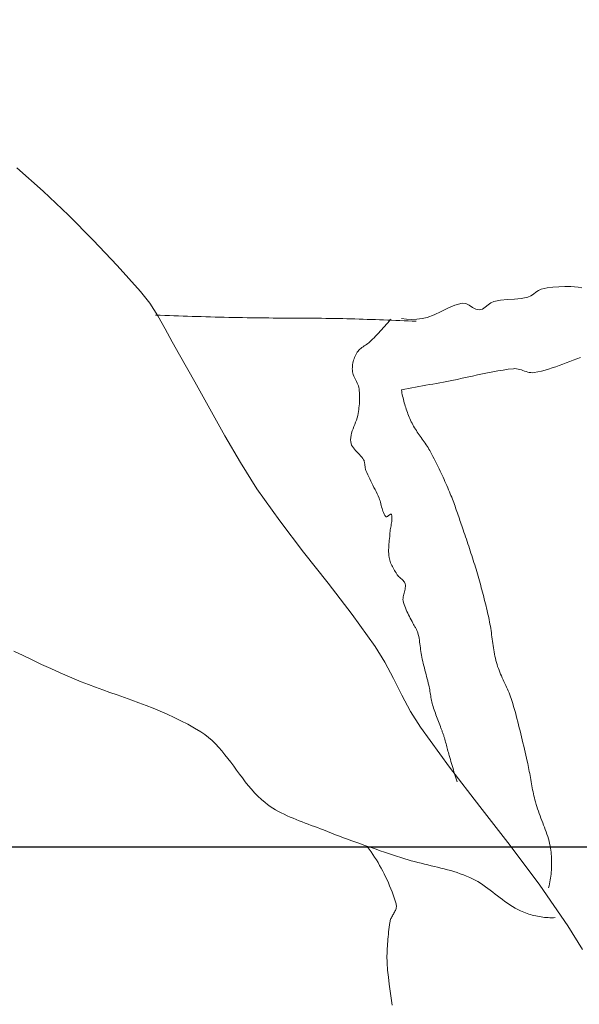
# Model space of a CAD drawing. Units: inches. Extents: x 1484 to 2008, y 1843 to 2590.
# Tile 7 of 21: x 1853 to 1872, y 2005 to 2039. Entities that reach past the tile are written whole.
import ezdxf

# ---------------------------------------------------------------- set-up
doc = ezdxf.new("R2010")
doc.units = ezdxf.units.IN
doc.layers.add('A-ANNO-DIMS', color=2, linetype='Continuous', lineweight=18)
doc.layers.add('A-FURN', color=8, linetype='Continuous', lineweight=18)
doc.styles.get("Standard").update_dxf_attribs({"font": 'arial.ttf'})
doc.dimstyles.new('ISO-25', dxfattribs={"dimtxt": 7, "dimasz": 2.5, "dimexe": 1.25, "dimexo": 0.625, "dimtad": 1, "dimdec": 0, "dimlunit": 3, "dimtxsty": 'Standard', "dimcen": 2.5, "dimadec": 0, "dimazin": 0, "dimtfac": 1, "dimtdec": 0, "dimtmove": 0, "dimatfit": 3, "dimfxl": 1, "dimarcsym": 0})

# ---------------------------------------------------------------- blocks, each defined once
blk = doc.blocks.new('BED-DOUBLE')
for p, q in [((4.353, 67.391), (4.375, 67.517)), ((27.04, 67.54), (26.237, 67.038)), ((4.326, 67.139), (4.333, 67.265)), ((4.331, 66.934), (4.326, 67.139)), ((4.333, 67.265), (4.353, 67.391)), ((6.802, 67.342), (6.757, 67.462)), ((6.847, 67.221), (6.802, 67.342)), ((6.893, 67.101), (6.847, 67.221)), ((4.338, 66.728), (4.331, 66.934)), ((6.939, 66.981), (6.893, 67.101)), ((6.985, 66.86), (6.939, 66.981)), ((7.03, 66.739), (6.985, 66.86)), ((26.237, 67.038), (24.84, 66.077)), ((4.352, 66.524), (4.338, 66.728)), ((4.377, 66.32), (4.352, 66.524)), ((7.073, 66.618), (7.03, 66.739)), ((7.115, 66.496), (7.073, 66.618)), ((7.154, 66.374), (7.115, 66.496)), ((23.776, 66.463), (23.709, 66.456)), ((23.844, 66.468), (23.776, 66.463)), ((23.912, 66.472), (23.844, 66.468)), ((23.981, 66.475), (23.912, 66.472)), ((24.049, 66.476), (23.981, 66.475)), ((24.117, 66.476), (24.049, 66.476)), ((24.186, 66.475), (24.117, 66.476)), ((24.254, 66.472), (24.186, 66.475)), ((24.322, 66.468), (24.254, 66.472)), ((24.39, 66.463), (24.322, 66.468)), ((24.458, 66.456), (24.39, 66.463)), ((25.954, 66.542), (25.951, 66.603)), ((25.954, 66.481), (25.954, 66.542)), ((25.954, 66.42), (25.954, 66.481)), ((4.417, 66.12), (4.377, 66.32)), ((7.19, 66.251), (7.154, 66.374)), ((7.222, 66.127), (7.19, 66.251)), ((7.25, 66.002), (7.222, 66.127)), ((22.62, 66.141), (22.542, 66.111)), ((22.698, 66.172), (22.62, 66.141)), ((22.777, 66.202), (22.698, 66.172)), ((22.855, 66.232), (22.777, 66.202)), ((22.933, 66.261), (22.855, 66.232)), ((23.012, 66.289), (22.933, 66.261)), ((23.091, 66.316), (23.012, 66.289)), ((23.17, 66.342), (23.091, 66.316)), ((23.25, 66.366), (23.17, 66.342)), ((23.33, 66.387), (23.25, 66.366)), ((23.411, 66.407), (23.33, 66.387)), ((23.492, 66.424), (23.411, 66.407)), ((23.574, 66.438), (23.492, 66.424)), ((23.641, 66.448), (23.574, 66.438)), ((23.709, 66.456), (23.641, 66.448)), ((24.526, 66.448), (24.458, 66.456)), ((24.594, 66.439), (24.526, 66.448)), ((24.661, 66.428), (24.594, 66.439)), ((24.728, 66.416), (24.661, 66.428)), ((24.795, 66.403), (24.728, 66.416)), ((24.861, 66.388), (24.795, 66.403)), ((24.927, 66.372), (24.861, 66.388)), ((25.927, 66.114), (25.935, 66.175)), ((25.935, 66.175), (25.942, 66.236)), ((25.942, 66.236), (25.948, 66.298)), ((25.948, 66.298), (25.951, 66.359)), ((25.951, 66.359), (25.954, 66.42)), ((4.458, 66.023), (4.417, 66.12)), ((4.52, 65.935), (4.458, 66.023)), ((4.588, 65.85), (4.52, 65.935)), ((4.65, 65.762), (4.588, 65.85)), ((7.274, 65.876), (7.25, 66.002)), ((7.279, 65.821), (7.274, 65.876)), ((7.277, 65.767), (7.279, 65.821)), ((21.363, 65.788), (21.293, 65.775)), ((21.433, 65.801), (21.363, 65.788)), ((21.503, 65.814), (21.433, 65.801)), ((21.573, 65.827), (21.503, 65.814)), ((21.642, 65.841), (21.573, 65.827)), ((21.712, 65.856), (21.642, 65.841)), ((21.781, 65.871), (21.712, 65.856)), ((21.851, 65.887), (21.781, 65.871)), ((21.92, 65.904), (21.851, 65.887)), ((21.988, 65.921), (21.92, 65.904)), ((22.069, 65.944), (21.988, 65.921)), ((22.148, 65.969), (22.069, 65.944)), ((22.228, 65.995), (22.148, 65.969)), ((22.307, 66.022), (22.228, 65.995)), ((22.385, 66.051), (22.307, 66.022)), ((22.464, 66.081), (22.385, 66.051)), ((22.542, 66.111), (22.464, 66.081)), ((24.84, 66.077), (23.483, 65.057)), ((25.847, 65.754), (25.864, 65.813)), ((25.864, 65.813), (25.88, 65.872)), ((25.88, 65.872), (25.894, 65.932)), ((25.894, 65.932), (25.906, 65.993)), ((25.906, 65.993), (25.917, 66.053)), ((25.917, 66.053), (25.927, 66.114)), ((4.692, 65.665), (4.65, 65.762)), ((4.735, 65.435), (4.692, 65.665)), ((7.186, 65.439), (7.205, 65.494)), ((7.205, 65.494), (7.224, 65.548)), ((7.224, 65.548), (7.242, 65.603)), ((7.242, 65.603), (7.257, 65.658)), ((7.257, 65.658), (7.27, 65.712)), ((7.27, 65.712), (7.277, 65.767)), ((19.863, 65.47), (19.758, 65.445)), ((19.967, 65.495), (19.863, 65.47)), ((20.072, 65.519), (19.967, 65.495)), ((20.176, 65.543), (20.072, 65.519)), ((20.281, 65.568), (20.176, 65.543)), ((20.385, 65.592), (20.281, 65.568)), ((20.49, 65.616), (20.385, 65.592)), ((20.594, 65.64), (20.49, 65.616)), ((20.664, 65.656), (20.594, 65.64)), ((20.733, 65.671), (20.664, 65.656)), ((20.803, 65.685), (20.733, 65.671)), ((20.873, 65.699), (20.803, 65.685)), ((20.943, 65.712), (20.873, 65.699)), ((21.013, 65.725), (20.943, 65.712)), ((21.083, 65.738), (21.013, 65.725)), ((21.153, 65.751), (21.083, 65.738)), ((21.223, 65.763), (21.153, 65.751)), ((21.293, 65.775), (21.223, 65.763)), ((25.717, 65.411), (25.742, 65.466)), ((25.742, 65.466), (25.766, 65.522)), ((25.766, 65.522), (25.788, 65.579)), ((25.788, 65.579), (25.809, 65.637)), ((25.809, 65.637), (25.829, 65.695)), ((25.829, 65.695), (25.847, 65.754)), ((4.756, 65.2), (4.735, 65.435)), ((4.771, 64.964), (4.756, 65.2)), ((7.141, 65.22), (7.146, 65.275)), ((7.143, 65.165), (7.141, 65.22)), ((7.163, 64.987), (7.143, 65.165)), ((7.146, 65.275), (7.156, 65.33)), ((7.156, 65.33), (7.17, 65.385)), ((7.17, 65.385), (7.186, 65.439)), ((18.515, 65.112), (18.448, 65.09)), ((18.617, 65.143), (18.515, 65.112)), ((18.72, 65.174), (18.617, 65.143)), ((18.823, 65.204), (18.72, 65.174)), ((18.926, 65.233), (18.823, 65.204)), ((19.03, 65.261), (18.926, 65.233)), ((19.133, 65.289), (19.03, 65.261)), ((19.237, 65.316), (19.133, 65.289)), ((19.341, 65.343), (19.237, 65.316)), ((19.445, 65.369), (19.341, 65.343)), ((19.549, 65.395), (19.445, 65.369)), ((19.654, 65.42), (19.549, 65.395)), ((19.758, 65.445), (19.654, 65.42)), ((25.512, 65.049), (25.568, 65.137)), ((25.568, 65.137), (25.621, 65.226)), ((25.621, 65.226), (25.67, 65.318)), ((25.67, 65.318), (25.717, 65.411)), ((4.792, 64.729), (4.771, 64.964)), ((7.188, 64.811), (7.163, 64.987)), ((7.216, 64.634), (7.188, 64.811)), ((17.735, 64.785), (17.67, 64.757)), ((17.799, 64.815), (17.735, 64.785)), ((17.863, 64.844), (17.799, 64.815)), ((17.927, 64.873), (17.863, 64.844)), ((17.992, 64.903), (17.927, 64.873)), ((18.056, 64.932), (17.992, 64.903)), ((18.12, 64.961), (18.056, 64.932)), ((18.185, 64.989), (18.12, 64.961)), ((18.25, 65.016), (18.185, 64.989)), ((18.316, 65.042), (18.25, 65.016)), ((18.381, 65.067), (18.316, 65.042)), ((18.448, 65.09), (18.381, 65.067)), ((23.483, 65.057), (22.143, 64.011)), ((25.268, 64.709), (25.331, 64.793)), ((25.331, 64.793), (25.393, 64.877)), ((25.393, 64.877), (25.453, 64.963)), ((25.453, 64.963), (25.512, 65.049)), ((4.836, 64.499), (4.792, 64.729)), ((4.884, 64.393), (4.836, 64.499)), ((7.248, 64.459), (7.216, 64.634)), ((7.282, 64.283), (7.248, 64.459)), ((16.408, 64.44), (16.334, 64.43)), ((16.482, 64.45), (16.408, 64.44)), ((16.555, 64.46), (16.482, 64.45)), ((16.629, 64.47), (16.555, 64.46)), ((16.702, 64.481), (16.629, 64.47)), ((16.775, 64.492), (16.702, 64.481)), ((16.848, 64.505), (16.775, 64.492)), ((16.921, 64.518), (16.848, 64.505)), ((16.993, 64.533), (16.921, 64.518)), ((17.066, 64.549), (16.993, 64.533)), ((17.138, 64.567), (17.066, 64.549)), ((17.209, 64.586), (17.138, 64.567)), ((17.277, 64.606), (17.209, 64.586)), ((17.343, 64.627), (17.277, 64.606)), ((17.41, 64.651), (17.343, 64.627)), ((17.475, 64.676), (17.41, 64.651)), ((17.541, 64.702), (17.475, 64.676)), ((17.606, 64.729), (17.541, 64.702)), ((17.67, 64.757), (17.606, 64.729)), ((25.013, 64.375), (25.077, 64.458)), ((25.077, 64.458), (25.141, 64.542)), ((25.141, 64.542), (25.205, 64.625)), ((25.205, 64.625), (25.268, 64.709)), ((4.957, 64.296), (4.884, 64.393)), ((5.035, 64.202), (4.957, 64.296)), ((5.098, 64.104), (5.035, 64.202)), ((5.128, 63.995), (5.098, 64.104)), ((7.317, 64.108), (7.282, 64.283)), ((7.355, 63.934), (7.317, 64.108)), ((14.802, 64.109), (14.723, 64.088)), ((14.88, 64.129), (14.802, 64.109)), ((14.959, 64.15), (14.88, 64.129)), ((15.038, 64.17), (14.959, 64.15)), ((15.116, 64.189), (15.038, 64.17)), ((15.195, 64.209), (15.116, 64.189)), ((15.274, 64.228), (15.195, 64.209)), ((15.353, 64.247), (15.274, 64.228)), ((15.432, 64.265), (15.353, 64.247)), ((15.511, 64.283), (15.432, 64.265)), ((15.59, 64.301), (15.511, 64.283)), ((15.669, 64.319), (15.59, 64.301)), ((15.749, 64.336), (15.669, 64.319)), ((15.821, 64.351), (15.749, 64.336)), ((15.894, 64.364), (15.821, 64.351)), ((15.967, 64.377), (15.894, 64.364)), ((16.04, 64.389), (15.967, 64.377)), ((16.114, 64.4), (16.04, 64.389)), ((16.187, 64.41), (16.114, 64.4)), ((16.261, 64.42), (16.187, 64.41)), ((16.334, 64.43), (16.261, 64.42)), ((24.773, 64.033), (24.83, 64.12)), ((24.83, 64.12), (24.89, 64.206)), ((24.89, 64.206), (24.951, 64.291)), ((24.951, 64.291), (25.013, 64.375)), ((5.042, 63.759), (5.105, 63.874)), ((5.105, 63.874), (5.128, 63.995)), ((7.393, 63.759), (7.355, 63.934)), ((13.618, 63.764), (13.539, 63.738)), ((13.698, 63.789), (13.618, 63.764)), ((13.777, 63.814), (13.698, 63.789)), ((13.857, 63.839), (13.777, 63.814)), ((13.937, 63.864), (13.857, 63.839)), ((14.016, 63.888), (13.937, 63.864)), ((14.096, 63.912), (14.016, 63.888)), ((14.176, 63.935), (14.096, 63.912)), ((14.254, 63.958), (14.176, 63.935)), ((14.332, 63.98), (14.254, 63.958)), ((14.41, 64.002), (14.332, 63.98)), ((14.489, 64.024), (14.41, 64.002)), ((14.567, 64.045), (14.489, 64.024)), ((14.645, 64.067), (14.567, 64.045)), ((14.723, 64.088), (14.645, 64.067)), ((22.143, 64.011), (20.798, 62.974)), ((24.573, 63.669), (24.617, 63.763)), ((24.617, 63.763), (24.666, 63.855)), ((24.666, 63.855), (24.718, 63.945)), ((24.718, 63.945), (24.773, 64.033)), ((4.895, 63.413), (4.909, 63.533)), ((4.909, 63.533), (4.967, 63.647)), ((4.967, 63.647), (5.042, 63.759)), ((7.432, 63.584), (7.393, 63.759)), ((7.47, 63.41), (7.432, 63.584)), ((12.669, 63.446), (12.59, 63.419)), ((12.748, 63.472), (12.669, 63.446)), ((12.827, 63.499), (12.748, 63.472)), ((12.906, 63.526), (12.827, 63.499)), ((12.985, 63.553), (12.906, 63.526)), ((13.064, 63.58), (12.985, 63.553)), ((13.143, 63.607), (13.064, 63.58)), ((13.222, 63.633), (13.143, 63.607)), ((13.301, 63.66), (13.222, 63.633)), ((13.381, 63.686), (13.301, 63.66)), ((13.46, 63.712), (13.381, 63.686)), ((13.539, 63.738), (13.46, 63.712)), ((24.445, 63.347), (24.484, 63.456)), ((24.484, 63.456), (24.527, 63.563)), ((24.527, 63.563), (24.573, 63.669)), ((4.96, 63.162), (4.895, 63.413)), ((5.064, 62.923), (4.96, 63.162)), ((7.507, 63.235), (7.47, 63.41)), ((7.543, 63.06), (7.507, 63.235)), ((11.668, 63.098), (11.607, 63.074)), ((11.729, 63.12), (11.668, 63.098)), ((11.79, 63.143), (11.729, 63.12)), ((11.851, 63.165), (11.79, 63.143)), ((11.912, 63.187), (11.851, 63.165)), ((11.974, 63.209), (11.912, 63.187)), ((12.035, 63.23), (11.974, 63.209)), ((12.097, 63.251), (12.035, 63.23)), ((12.158, 63.272), (12.097, 63.251)), ((12.22, 63.293), (12.158, 63.272)), ((12.282, 63.314), (12.22, 63.293)), ((12.344, 63.335), (12.282, 63.314)), ((12.405, 63.356), (12.344, 63.335)), ((12.467, 63.377), (12.405, 63.356)), ((12.529, 63.398), (12.467, 63.377)), ((12.59, 63.419), (12.529, 63.398)), ((20.812, 63.088), (20.743, 63.068)), ((20.881, 63.109), (20.812, 63.088)), ((20.95, 63.13), (20.881, 63.109)), ((21.019, 63.151), (20.95, 63.13)), ((21.088, 63.172), (21.019, 63.151)), ((21.158, 63.193), (21.088, 63.172)), ((21.227, 63.214), (21.158, 63.193)), ((21.296, 63.235), (21.227, 63.214)), ((24.34, 63.017), (24.373, 63.128)), ((24.373, 63.128), (24.408, 63.238)), ((24.408, 63.238), (24.445, 63.347)), ((5.185, 62.688), (5.064, 62.923)), ((7.577, 62.885), (7.543, 63.06)), ((7.6, 62.765), (7.577, 62.885)), ((7.622, 62.645), (7.6, 62.765)), ((10.862, 62.755), (10.791, 62.722)), ((10.934, 62.788), (10.862, 62.755)), ((11.005, 62.82), (10.934, 62.788)), ((11.077, 62.852), (11.005, 62.82)), ((11.149, 62.884), (11.077, 62.852)), ((11.221, 62.915), (11.149, 62.884)), ((11.293, 62.946), (11.221, 62.915)), ((11.365, 62.977), (11.293, 62.946)), ((11.425, 63.002), (11.365, 62.977)), ((11.486, 63.027), (11.425, 63.002)), ((11.546, 63.051), (11.486, 63.027)), ((11.607, 63.074), (11.546, 63.051)), ((20.798, 62.974), (19.423, 61.978)), ((19.635, 62.75), (19.608, 62.74)), ((19.661, 62.759), (19.635, 62.75)), ((19.688, 62.768), (19.661, 62.759)), ((19.714, 62.777), (19.688, 62.768)), ((19.741, 62.785), (19.714, 62.777)), ((19.791, 62.8), (19.741, 62.785)), ((19.841, 62.815), (19.791, 62.8)), ((19.892, 62.829), (19.841, 62.815)), ((19.942, 62.843), (19.892, 62.829)), ((19.992, 62.857), (19.942, 62.843)), ((20.043, 62.87), (19.992, 62.857)), ((20.093, 62.883), (20.043, 62.87)), ((20.144, 62.897), (20.093, 62.883)), ((20.194, 62.91), (20.144, 62.897)), ((20.245, 62.924), (20.194, 62.91)), ((20.295, 62.938), (20.245, 62.924)), ((20.346, 62.952), (20.295, 62.938)), ((20.396, 62.966), (20.346, 62.952)), ((20.465, 62.986), (20.396, 62.966)), ((20.535, 63.006), (20.465, 62.986)), ((20.604, 63.027), (20.535, 63.006)), ((20.673, 63.047), (20.604, 63.027)), ((20.743, 63.068), (20.673, 63.047)), ((24.252, 62.681), (24.28, 62.794)), ((24.28, 62.794), (24.309, 62.906)), ((24.309, 62.906), (24.34, 63.017)), ((5.3, 62.451), (5.185, 62.688)), ((5.386, 62.205), (5.3, 62.451)), ((7.644, 62.525), (7.622, 62.645)), ((7.667, 62.405), (7.644, 62.525)), ((10.226, 62.447), (10.156, 62.41)), ((10.296, 62.482), (10.226, 62.447)), ((10.366, 62.518), (10.296, 62.482)), ((10.436, 62.553), (10.366, 62.518)), ((10.507, 62.587), (10.436, 62.553)), ((10.577, 62.622), (10.507, 62.587)), ((10.648, 62.656), (10.577, 62.622)), ((10.719, 62.689), (10.648, 62.656)), ((10.791, 62.722), (10.719, 62.689)), ((18.721, 62.413), (18.663, 62.396)), ((18.778, 62.431), (18.721, 62.413)), ((18.835, 62.45), (18.778, 62.431)), ((18.892, 62.47), (18.835, 62.45)), ((18.948, 62.491), (18.892, 62.47)), ((19.005, 62.512), (18.948, 62.491)), ((19.061, 62.533), (19.005, 62.512)), ((19.117, 62.555), (19.061, 62.533)), ((19.173, 62.577), (19.117, 62.555)), ((19.229, 62.598), (19.173, 62.577)), ((19.285, 62.62), (19.229, 62.598)), ((19.342, 62.641), (19.285, 62.62)), ((19.398, 62.662), (19.342, 62.641)), ((19.425, 62.671), (19.398, 62.662)), ((19.451, 62.681), (19.425, 62.671)), ((19.477, 62.691), (19.451, 62.681)), ((19.503, 62.701), (19.477, 62.691)), ((19.53, 62.711), (19.503, 62.701)), ((19.556, 62.721), (19.53, 62.711)), ((19.582, 62.73), (19.556, 62.721)), ((19.608, 62.74), (19.582, 62.73)), ((24.171, 62.343), (24.197, 62.456)), ((24.197, 62.456), (24.224, 62.569)), ((24.224, 62.569), (24.252, 62.681)), ((5.422, 62.034), (5.386, 62.205)), ((7.689, 62.285), (7.667, 62.405)), ((7.711, 62.166), (7.689, 62.285)), ((7.733, 62.046), (7.711, 62.166)), ((9.601, 62.077), (9.553, 62.043)), ((9.65, 62.111), (9.601, 62.077)), ((9.698, 62.145), (9.65, 62.111)), ((9.747, 62.178), (9.698, 62.145)), ((9.797, 62.21), (9.747, 62.178)), ((9.846, 62.241), (9.797, 62.21)), ((9.897, 62.271), (9.846, 62.241)), ((9.948, 62.3), (9.897, 62.271)), ((10.017, 62.337), (9.948, 62.3)), ((10.087, 62.374), (10.017, 62.337)), ((10.156, 62.41), (10.087, 62.374)), ((17.248, 62.078), (17.174, 62.06)), ((17.322, 62.096), (17.248, 62.078)), ((17.397, 62.115), (17.322, 62.096)), ((17.471, 62.134), (17.397, 62.115)), ((17.545, 62.153), (17.471, 62.134)), ((17.619, 62.173), (17.545, 62.153)), ((17.693, 62.192), (17.619, 62.173)), ((17.767, 62.211), (17.693, 62.192)), ((17.842, 62.23), (17.767, 62.211)), ((17.916, 62.247), (17.842, 62.23)), ((17.991, 62.265), (17.916, 62.247)), ((18.042, 62.276), (17.991, 62.265)), ((18.094, 62.286), (18.042, 62.276)), ((18.146, 62.296), (18.094, 62.286)), ((18.198, 62.305), (18.146, 62.296)), ((18.25, 62.313), (18.198, 62.305)), ((18.302, 62.322), (18.25, 62.313)), ((18.354, 62.331), (18.302, 62.322)), ((18.406, 62.34), (18.354, 62.331)), ((18.458, 62.349), (18.406, 62.34)), ((18.509, 62.359), (18.458, 62.349)), ((18.561, 62.371), (18.509, 62.359)), ((18.612, 62.383), (18.561, 62.371)), ((18.663, 62.396), (18.612, 62.383)), ((24.09, 62.004), (24.118, 62.116)), ((24.118, 62.116), (24.144, 62.229)), ((24.144, 62.229), (24.171, 62.343)), ((5.444, 61.859), (5.422, 62.034)), ((5.451, 61.683), (5.444, 61.859)), ((5.512, 61.697), (5.518, 61.837)), ((7.755, 61.926), (7.733, 62.046)), ((7.776, 61.806), (7.755, 61.926)), ((7.798, 61.686), (7.776, 61.806)), ((9.114, 61.747), (9.063, 61.719)), ((9.165, 61.777), (9.114, 61.747)), ((9.214, 61.808), (9.165, 61.777)), ((9.264, 61.84), (9.214, 61.808)), ((9.313, 61.873), (9.264, 61.84)), ((9.361, 61.907), (9.313, 61.873)), ((9.409, 61.94), (9.361, 61.907)), ((9.457, 61.975), (9.409, 61.94)), ((9.505, 62.009), (9.457, 61.975)), ((9.553, 62.043), (9.505, 62.009)), ((15.912, 61.745), (15.887, 61.731)), ((15.937, 61.759), (15.912, 61.745)), ((15.961, 61.774), (15.937, 61.759)), ((15.985, 61.789), (15.961, 61.774)), ((16.01, 61.805), (15.985, 61.789)), ((16.034, 61.82), (16.01, 61.805)), ((16.058, 61.835), (16.034, 61.82)), ((16.083, 61.848), (16.058, 61.835)), ((16.108, 61.861), (16.083, 61.848)), ((16.134, 61.873), (16.108, 61.861)), ((16.16, 61.883), (16.134, 61.873)), ((16.187, 61.891), (16.16, 61.883)), ((16.25, 61.907), (16.187, 61.891)), ((16.314, 61.92), (16.25, 61.907)), ((16.378, 61.932), (16.314, 61.92)), ((16.443, 61.943), (16.378, 61.932)), ((16.507, 61.952), (16.443, 61.943)), ((16.572, 61.961), (16.507, 61.952)), ((16.637, 61.969), (16.572, 61.961)), ((16.702, 61.977), (16.637, 61.969)), ((16.766, 61.985), (16.702, 61.977)), ((16.831, 61.994), (16.766, 61.985)), ((16.896, 62.004), (16.831, 61.994)), ((16.96, 62.015), (16.896, 62.004)), ((17.024, 62.027), (16.96, 62.015)), ((17.099, 62.043), (17.024, 62.027)), ((17.174, 62.06), (17.099, 62.043)), ((19.423, 61.978), (18.885, 61.644)), ((24.002, 61.667), (24.033, 61.779)), ((24.033, 61.779), (24.062, 61.891)), ((24.062, 61.891), (24.09, 62.004)), ((5.424, 61.333), (5.445, 61.507)), ((5.445, 61.507), (5.451, 61.683)), ((5.493, 61.277), (5.499, 61.417)), ((5.499, 61.417), (5.505, 61.557)), ((5.505, 61.557), (5.512, 61.697)), ((7.82, 61.566), (7.798, 61.686)), ((7.841, 61.446), (7.82, 61.566)), ((7.863, 61.326), (7.841, 61.446)), ((8.256, 61.411), (8.2, 61.396)), ((8.312, 61.426), (8.256, 61.411)), ((8.367, 61.442), (8.312, 61.426)), ((8.422, 61.459), (8.367, 61.442)), ((8.477, 61.476), (8.422, 61.459)), ((8.532, 61.494), (8.477, 61.476)), ((8.586, 61.513), (8.532, 61.494)), ((8.64, 61.533), (8.586, 61.513)), ((8.694, 61.553), (8.64, 61.533)), ((8.748, 61.574), (8.694, 61.553)), ((8.801, 61.596), (8.748, 61.574)), ((8.854, 61.619), (8.801, 61.596)), ((8.906, 61.642), (8.854, 61.619)), ((8.958, 61.666), (8.906, 61.642)), ((9.011, 61.691), (8.958, 61.666)), ((9.063, 61.719), (9.011, 61.691)), ((14.428, 61.411), (14.401, 61.39)), ((14.455, 61.43), (14.428, 61.411)), ((14.485, 61.445), (14.455, 61.43)), ((14.517, 61.455), (14.485, 61.445)), ((14.561, 61.462), (14.517, 61.455)), ((14.605, 61.463), (14.561, 61.462)), ((14.649, 61.46), (14.605, 61.463)), ((14.694, 61.452), (14.649, 61.46)), ((14.738, 61.442), (14.694, 61.452)), ((14.783, 61.43), (14.738, 61.442)), ((14.828, 61.418), (14.783, 61.43)), ((14.873, 61.405), (14.828, 61.418)), ((14.918, 61.395), (14.873, 61.405)), ((15.158, 61.401), (15.095, 61.387)), ((15.219, 61.419), (15.158, 61.401)), ((15.28, 61.439), (15.219, 61.419)), ((15.339, 61.462), (15.28, 61.439)), ((15.399, 61.488), (15.339, 61.462)), ((15.457, 61.515), (15.399, 61.488)), ((15.515, 61.543), (15.457, 61.515)), ((15.573, 61.573), (15.515, 61.543)), ((15.631, 61.602), (15.573, 61.573)), ((15.688, 61.632), (15.631, 61.602)), ((15.746, 61.662), (15.688, 61.632)), ((15.804, 61.691), (15.746, 61.662)), ((15.862, 61.719), (15.804, 61.691)), ((15.887, 61.731), (15.862, 61.719)), ((18.885, 61.644), (18.326, 61.345)), ((23.889, 61.305), (23.935, 61.445)), ((23.935, 61.445), (23.969, 61.556)), ((23.969, 61.556), (24.002, 61.667)), ((5.482, 60.997), (5.487, 61.137)), ((5.487, 61.137), (5.493, 61.277)), ((7.919, 61.336), (7.863, 61.326)), ((7.976, 61.346), (7.919, 61.336)), ((8.032, 61.358), (7.976, 61.346)), ((8.088, 61.37), (8.032, 61.358)), ((8.144, 61.383), (8.088, 61.37)), ((8.2, 61.396), (8.144, 61.383)), ((14.01, 61.067), (13.968, 61.043)), ((14.053, 61.091), (14.01, 61.067)), ((14.095, 61.116), (14.053, 61.091)), ((14.136, 61.142), (14.095, 61.116)), ((14.178, 61.167), (14.136, 61.142)), ((14.206, 61.186), (14.178, 61.167)), ((14.233, 61.208), (14.206, 61.186)), ((14.258, 61.233), (14.233, 61.208)), ((14.282, 61.259), (14.258, 61.233)), ((14.306, 61.286), (14.282, 61.259)), ((14.329, 61.313), (14.306, 61.286)), ((14.353, 61.34), (14.329, 61.313)), ((14.377, 61.366), (14.353, 61.34)), ((14.401, 61.39), (14.377, 61.366)), ((14.962, 61.386), (14.918, 61.395)), ((15.007, 61.382), (14.962, 61.386)), ((15.051, 61.381), (15.007, 61.382)), ((15.095, 61.387), (15.051, 61.381)), ((18.326, 61.345), (17.758, 61.059)), ((23.797, 61.023), (23.843, 61.164)), ((23.843, 61.164), (23.889, 61.305)), ((25.272, 61.079), (25.168, 61.043)), ((25.377, 61.113), (25.272, 61.079)), ((25.483, 61.145), (25.377, 61.113)), ((25.515, 61.153), (25.483, 61.145)), ((25.546, 61.155), (25.515, 61.153)), ((25.578, 61.154), (25.546, 61.155)), ((25.609, 61.15), (25.578, 61.154)), ((25.64, 61.142), (25.609, 61.15)), ((25.671, 61.132), (25.64, 61.142)), ((25.703, 61.12), (25.671, 61.132)), ((25.734, 61.105), (25.703, 61.12)), ((25.765, 61.089), (25.734, 61.105)), ((25.796, 61.072), (25.765, 61.089)), ((25.827, 61.054), (25.796, 61.072)), ((5.509, 60.905), (5.449, 60.954)), ((5.471, 60.716), (5.476, 60.856)), ((5.476, 60.856), (5.482, 60.997)), ((5.568, 60.856), (5.509, 60.905)), ((5.627, 60.806), (5.568, 60.856)), ((5.685, 60.755), (5.627, 60.806)), ((5.743, 60.704), (5.685, 60.755)), ((12.122, 60.735), (12.075, 60.714)), ((12.167, 60.76), (12.122, 60.735)), ((12.128, 60.979), (12.125, 60.969)), ((12.125, 60.969), (12.128, 60.957)), ((12.139, 60.985), (12.128, 60.979)), ((12.128, 60.957), (12.136, 60.941)), ((12.136, 60.941), (12.148, 60.924)), ((12.186, 60.995), (12.139, 60.985)), ((12.148, 60.924), (12.162, 60.906)), ((12.162, 60.906), (12.177, 60.887)), ((12.21, 60.789), (12.167, 60.76)), ((12.177, 60.887), (12.192, 60.867)), ((12.233, 61), (12.186, 60.995)), ((12.192, 60.867), (12.205, 60.848)), ((12.205, 60.848), (12.215, 60.831)), ((12.218, 60.8), (12.21, 60.789)), ((12.215, 60.831), (12.219, 60.814)), ((12.219, 60.814), (12.218, 60.8)), ((12.281, 61.001), (12.233, 61)), ((12.329, 60.999), (12.281, 61.001)), ((12.377, 60.995), (12.329, 60.999)), ((12.426, 60.988), (12.377, 60.995)), ((12.474, 60.98), (12.426, 60.988)), ((12.523, 60.971), (12.474, 60.98)), ((12.572, 60.961), (12.523, 60.971)), ((12.621, 60.953), (12.572, 60.961)), ((12.669, 60.945), (12.621, 60.953)), ((12.718, 60.939), (12.669, 60.945)), ((12.766, 60.935), (12.718, 60.939)), ((12.831, 60.93), (12.766, 60.935)), ((12.896, 60.925), (12.831, 60.93)), ((12.961, 60.919), (12.896, 60.925)), ((13.026, 60.912), (12.961, 60.919)), ((13.091, 60.906), (13.026, 60.912)), ((13.156, 60.9), (13.091, 60.906)), ((13.221, 60.895), (13.156, 60.9)), ((13.285, 60.891), (13.221, 60.895)), ((13.35, 60.889), (13.285, 60.891)), ((13.415, 60.889), (13.35, 60.889)), ((13.479, 60.892), (13.415, 60.889)), ((13.543, 60.897), (13.479, 60.892)), ((13.607, 60.906), (13.543, 60.897)), ((13.655, 60.915), (13.607, 60.906)), ((13.701, 60.927), (13.655, 60.915)), ((13.747, 60.942), (13.701, 60.927)), ((13.792, 60.958), (13.747, 60.942)), ((13.837, 60.977), (13.792, 60.958)), ((13.881, 60.998), (13.837, 60.977)), ((13.925, 61.019), (13.881, 60.998)), ((13.968, 61.043), (13.925, 61.019)), ((17.198, 60.761), (16.659, 60.428)), ((17.758, 61.059), (17.198, 60.761)), ((23.657, 60.601), (23.704, 60.742)), ((23.704, 60.742), (23.751, 60.882)), ((23.751, 60.882), (23.797, 61.023)), ((24.455, 60.738), (24.356, 60.687)), ((24.554, 60.787), (24.455, 60.738)), ((24.655, 60.834), (24.554, 60.787)), ((24.756, 60.879), (24.655, 60.834)), ((24.858, 60.923), (24.756, 60.879)), ((24.961, 60.965), (24.858, 60.923)), ((25.064, 61.005), (24.961, 60.965)), ((25.168, 61.043), (25.064, 61.005)), ((25.858, 61.036), (25.827, 61.054)), ((25.889, 61.018), (25.858, 61.036)), ((25.921, 61.001), (25.889, 61.018)), ((25.952, 60.985), (25.921, 61.001)), ((25.984, 60.969), (25.952, 60.985)), ((26.016, 60.956), (25.984, 60.969)), ((26.049, 60.945), (26.016, 60.956)), ((26.081, 60.936), (26.049, 60.945)), ((26.114, 60.93), (26.081, 60.936)), ((26.195, 60.92), (26.114, 60.93)), ((26.277, 60.91), (26.195, 60.92)), ((26.358, 60.9), (26.277, 60.91)), ((26.44, 60.89), (26.358, 60.9)), ((26.521, 60.881), (26.44, 60.89)), ((26.603, 60.873), (26.521, 60.881)), ((26.685, 60.865), (26.603, 60.873)), ((26.766, 60.858), (26.685, 60.865)), ((26.848, 60.851), (26.766, 60.858)), ((26.93, 60.846), (26.848, 60.851)), ((27.012, 60.841), (26.93, 60.846)), ((27.094, 60.837), (27.012, 60.841)), ((27.176, 60.835), (27.094, 60.837)), ((27.258, 60.833), (27.176, 60.835)), ((27.339, 60.833), (27.258, 60.833)), ((27.421, 60.834), (27.339, 60.833)), ((27.503, 60.837), (27.421, 60.834)), ((27.585, 60.841), (27.503, 60.837)), ((27.666, 60.847), (27.585, 60.841)), ((27.747, 60.854), (27.666, 60.847)), ((27.988, 60.881), (27.747, 60.854)), ((28.227, 60.91), (27.988, 60.881)), ((28.467, 60.943), (28.227, 60.91)), ((28.706, 60.978), (28.467, 60.943)), ((28.945, 61.015), (28.706, 60.978)), ((5.456, 60.296), (5.461, 60.436)), ((5.461, 60.436), (5.466, 60.576)), ((5.466, 60.576), (5.471, 60.716)), ((5.8, 60.653), (5.743, 60.704)), ((5.857, 60.601), (5.8, 60.653)), ((5.914, 60.548), (5.857, 60.601)), ((5.97, 60.496), (5.914, 60.548)), ((6.026, 60.442), (5.97, 60.496)), ((6.081, 60.389), (6.026, 60.442)), ((6.136, 60.335), (6.081, 60.389)), ((11.281, 60.422), (11.209, 60.386)), ((11.353, 60.458), (11.281, 60.422)), ((11.426, 60.493), (11.353, 60.458)), ((11.499, 60.527), (11.426, 60.493)), ((11.573, 60.559), (11.499, 60.527)), ((11.621, 60.579), (11.573, 60.559)), ((11.671, 60.595), (11.621, 60.579)), ((11.721, 60.61), (11.671, 60.595)), ((11.773, 60.624), (11.721, 60.61)), ((11.824, 60.637), (11.773, 60.624)), ((11.876, 60.65), (11.824, 60.637)), ((11.927, 60.664), (11.876, 60.65)), ((11.977, 60.679), (11.927, 60.664)), ((12.027, 60.695), (11.977, 60.679)), ((12.075, 60.714), (12.027, 60.695)), ((16.659, 60.428), (15.564, 59.638)), ((23.562, 60.321), (23.61, 60.461)), ((23.61, 60.461), (23.657, 60.601)), ((23.876, 60.409), (23.784, 60.349)), ((23.97, 60.468), (23.876, 60.409)), ((24.065, 60.525), (23.97, 60.468)), ((24.161, 60.581), (24.065, 60.525)), ((24.258, 60.635), (24.161, 60.581)), ((24.356, 60.687), (24.258, 60.635)), ((5.447, 60.015), (5.452, 60.156)), ((5.452, 60.156), (5.456, 60.296)), ((6.191, 60.28), (6.136, 60.335)), ((6.223, 60.246), (6.191, 60.28)), ((6.253, 60.209), (6.223, 60.246)), ((6.281, 60.171), (6.253, 60.209)), ((6.308, 60.132), (6.281, 60.171)), ((6.335, 60.092), (6.308, 60.132)), ((6.362, 60.052), (6.335, 60.092)), ((6.389, 60.013), (6.362, 60.052)), ((10.319, 60.054), (10.293, 60.045)), ((10.346, 60.061), (10.319, 60.054)), ((10.374, 60.067), (10.346, 60.061)), ((10.402, 60.071), (10.374, 60.067)), ((10.431, 60.074), (10.402, 60.071)), ((10.46, 60.076), (10.431, 60.074)), ((10.489, 60.079), (10.46, 60.076)), ((10.517, 60.082), (10.489, 60.079)), ((10.546, 60.086), (10.517, 60.082)), ((10.574, 60.092), (10.546, 60.086)), ((10.601, 60.099), (10.574, 60.092)), ((10.628, 60.108), (10.601, 60.099)), ((10.702, 60.139), (10.628, 60.108)), ((10.776, 60.172), (10.702, 60.139)), ((10.849, 60.206), (10.776, 60.172)), ((10.921, 60.241), (10.849, 60.206)), ((10.993, 60.276), (10.921, 60.241)), ((11.065, 60.313), (10.993, 60.276)), ((11.137, 60.349), (11.065, 60.313)), ((11.209, 60.386), (11.137, 60.349)), ((23.465, 60.041), (23.514, 60.181)), ((23.602, 60.223), (23.513, 60.158)), ((23.514, 60.181), (23.562, 60.321)), ((23.692, 60.287), (23.602, 60.223)), ((23.784, 60.349), (23.692, 60.287)), ((5.435, 59.595), (5.439, 59.735)), ((5.439, 59.735), (5.443, 59.875)), ((5.443, 59.875), (5.447, 60.015)), ((6.416, 59.974), (6.389, 60.013)), ((6.445, 59.937), (6.416, 59.974)), ((6.476, 59.902), (6.445, 59.937)), ((6.508, 59.869), (6.476, 59.902)), ((6.543, 59.839), (6.508, 59.869)), ((6.581, 59.812), (6.543, 59.839)), ((6.623, 59.786), (6.581, 59.812)), ((6.667, 59.763), (6.623, 59.786)), ((6.712, 59.742), (6.667, 59.763)), ((6.757, 59.722), (6.712, 59.742)), ((6.804, 59.704), (6.757, 59.722)), ((7.443, 59.718), (7.395, 59.696)), ((7.49, 59.741), (7.443, 59.718)), ((7.538, 59.765), (7.49, 59.741)), ((7.586, 59.789), (7.538, 59.765)), ((7.634, 59.812), (7.586, 59.789)), ((7.682, 59.833), (7.634, 59.812)), ((7.731, 59.851), (7.682, 59.833)), ((7.781, 59.865), (7.731, 59.851)), ((7.832, 59.875), (7.781, 59.865)), ((7.896, 59.883), (7.832, 59.875)), ((7.961, 59.888), (7.896, 59.883)), ((8.026, 59.892), (7.961, 59.888)), ((8.09, 59.894), (8.026, 59.892)), ((8.155, 59.894), (8.09, 59.894)), ((8.22, 59.892), (8.155, 59.894)), ((8.285, 59.889), (8.22, 59.892)), ((8.35, 59.885), (8.285, 59.889)), ((8.415, 59.879), (8.35, 59.885)), ((8.48, 59.873), (8.415, 59.879)), ((8.545, 59.865), (8.48, 59.873)), ((8.609, 59.856), (8.545, 59.865)), ((8.673, 59.846), (8.609, 59.856)), ((8.75, 59.831), (8.673, 59.846)), ((8.825, 59.81), (8.75, 59.831)), ((8.901, 59.785), (8.825, 59.81)), ((8.976, 59.757), (8.901, 59.785)), ((9.05, 59.728), (8.976, 59.757)), ((9.125, 59.698), (9.05, 59.728)), ((9.903, 59.717), (9.858, 59.68)), ((9.948, 59.757), (9.903, 59.717)), ((9.992, 59.8), (9.948, 59.757)), ((10.035, 59.843), (9.992, 59.8)), ((10.079, 59.887), (10.035, 59.843)), ((10.123, 59.928), (10.079, 59.887)), ((10.169, 59.968), (10.123, 59.928)), ((10.217, 60.003), (10.169, 59.968)), ((10.267, 60.033), (10.217, 60.003)), ((10.293, 60.045), (10.267, 60.033)), ((23.317, 59.622), (23.367, 59.761)), ((23.367, 59.761), (23.416, 59.901)), ((23.416, 59.901), (23.465, 60.041)), ((5.428, 59.314), (5.432, 59.454)), ((5.432, 59.454), (5.435, 59.595)), ((6.852, 59.689), (6.804, 59.704)), ((6.9, 59.676), (6.852, 59.689)), ((6.949, 59.665), (6.9, 59.676)), ((6.998, 59.656), (6.949, 59.665)), ((7.047, 59.65), (6.998, 59.656)), ((7.097, 59.646), (7.047, 59.65)), ((7.146, 59.644), (7.097, 59.646)), ((7.195, 59.645), (7.146, 59.644)), ((7.246, 59.651), (7.195, 59.645)), ((7.297, 59.662), (7.246, 59.651)), ((7.346, 59.677), (7.297, 59.662)), ((7.395, 59.696), (7.346, 59.677)), ((9.199, 59.67), (9.125, 59.698)), ((9.273, 59.643), (9.199, 59.67)), ((9.348, 59.62), (9.273, 59.643)), ((9.423, 59.602), (9.348, 59.62)), ((9.499, 59.59), (9.423, 59.602)), ((9.575, 59.586), (9.499, 59.59)), ((9.652, 59.59), (9.575, 59.586)), ((9.708, 59.601), (9.652, 59.59)), ((9.76, 59.621), (9.708, 59.601)), ((9.81, 59.647), (9.76, 59.621)), ((9.858, 59.68), (9.81, 59.647)), ((15.564, 59.638), (14.493, 58.812)), ((23.215, 59.344), (23.266, 59.483)), ((23.266, 59.483), (23.317, 59.622)), ((5.422, 59.034), (5.425, 59.174)), ((5.425, 59.174), (5.428, 59.314)), ((23.057, 58.928), (23.11, 59.067)), ((23.11, 59.067), (23.163, 59.205)), ((23.163, 59.205), (23.215, 59.344)), ((5.415, 58.584), (5.417, 58.734)), ((5.417, 58.734), (5.419, 58.884)), ((5.419, 58.884), (5.422, 59.034)), ((14.493, 58.812), (13.43, 57.976)), ((22.948, 58.653), (23.003, 58.791)), ((23.003, 58.791), (23.057, 58.928)), ((5.412, 58.284), (5.413, 58.434)), ((5.413, 58.434), (5.415, 58.584)), ((22.828, 58.342), (22.867, 58.446)), ((22.867, 58.446), (22.907, 58.55)), ((22.907, 58.55), (22.948, 58.653)), ((5.41, 57.984), (5.411, 58.134)), ((5.411, 58.134), (5.412, 58.284)), ((22.671, 57.924), (22.711, 58.028)), ((22.711, 58.028), (22.75, 58.133)), ((22.75, 58.133), (22.789, 58.238)), ((22.789, 58.238), (22.828, 58.342)), ((5.409, 57.834), (5.41, 57.984)), ((5.409, 57.684), (5.409, 57.834)), ((13.43, 57.976), (12.356, 57.156)), ((22.547, 57.612), (22.59, 57.716)), ((22.59, 57.716), (22.631, 57.819)), ((22.631, 57.819), (22.671, 57.924)), ((5.407, 57.234), (5.408, 57.384)), ((5.408, 57.534), (5.409, 57.684)), ((5.408, 57.384), (5.408, 57.534)), ((22.411, 57.308), (22.459, 57.409)), ((22.459, 57.409), (22.504, 57.51)), ((22.504, 57.51), (22.547, 57.612)), ((5.406, 56.934), (5.407, 57.084)), ((5.407, 57.084), (5.407, 57.234)), ((12.356, 57.156), (11.254, 56.374)), ((22.199, 56.922), (22.256, 57.016)), ((22.256, 57.016), (22.31, 57.112)), ((22.31, 57.112), (22.362, 57.209)), ((22.362, 57.209), (22.411, 57.308)), ((5.404, 56.634), (5.405, 56.784)), ((5.405, 56.784), (5.406, 56.934)), ((22.008, 56.653), (22.075, 56.74)), ((22.075, 56.74), (22.139, 56.83)), ((22.139, 56.83), (22.199, 56.922)), ((5.401, 56.334), (5.402, 56.484)), ((5.402, 56.484), (5.404, 56.634)), ((11.254, 56.374), (10.361, 55.807)), ((21.673, 56.295), (21.791, 56.409)), ((21.791, 56.409), (21.903, 56.528)), ((21.903, 56.528), (22.008, 56.653)), ((5.393, 55.877), (5.396, 56.034)), ((5.396, 56.034), (5.399, 56.184)), ((5.399, 56.184), (5.401, 56.334)), ((21.296, 55.976), (21.425, 56.079)), ((21.425, 56.079), (21.551, 56.185)), ((21.551, 56.185), (21.673, 56.295)), ((5.387, 55.564), (5.39, 55.721)), ((5.39, 55.721), (5.393, 55.877)), ((10.361, 55.807), (9.446, 55.275)), ((20.762, 55.578), (20.896, 55.677)), ((20.896, 55.677), (21.031, 55.775)), ((21.031, 55.775), (21.164, 55.875)), ((21.164, 55.875), (21.296, 55.976)), ((5.38, 55.251), (5.383, 55.407)), ((5.383, 55.407), (5.387, 55.564)), ((20.367, 55.277), (20.497, 55.379)), ((20.497, 55.379), (20.629, 55.479)), ((20.629, 55.479), (20.762, 55.578)), ((5.372, 54.937), (5.376, 55.094)), ((5.376, 55.094), (5.38, 55.251)), ((9.446, 55.275), (8.519, 54.762)), ((20, 54.953), (20.118, 55.064)), ((20.118, 55.064), (20.24, 55.172)), ((20.24, 55.172), (20.367, 55.277)), ((5.364, 54.624), (5.368, 54.781)), ((5.368, 54.781), (5.372, 54.937)), ((8.519, 54.762), (7.591, 54.25)), ((19.681, 54.586), (19.781, 54.714)), ((19.781, 54.714), (19.887, 54.836)), ((19.887, 54.836), (20, 54.953)), ((5.355, 54.311), (5.359, 54.467)), ((5.359, 54.467), (5.364, 54.624)), ((19.454, 54.228), (19.59, 54.452)), ((19.59, 54.452), (19.681, 54.586)), ((5.34, 53.841), (5.345, 53.997)), ((5.345, 53.997), (5.35, 54.154)), ((5.35, 54.154), (5.355, 54.311)), ((7.591, 54.25), (6.672, 53.725)), ((19.205, 53.77), (19.326, 54.001)), ((19.326, 54.001), (19.454, 54.228)), ((5.33, 53.527), (5.335, 53.684)), ((5.335, 53.684), (5.34, 53.841)), ((6.672, 53.725), (6.226, 53.473)), ((19.091, 53.535), (19.205, 53.77)), ((5.319, 53.214), (5.325, 53.371)), ((5.325, 53.371), (5.33, 53.527)), ((6.226, 53.473), (5.774, 53.228)), ((18.982, 53.298), (19.091, 53.535)), ((5.328, 52.975), (4.899, 52.699)), ((5.308, 52.901), (5.313, 53.057)), ((5.313, 53.057), (5.319, 53.214)), ((5.774, 53.228), (5.328, 52.975)), ((18.778, 52.816), (18.878, 53.058)), ((18.878, 53.058), (18.982, 53.298)), ((4.899, 52.699), (4.496, 52.387)), ((18.683, 52.572), (18.778, 52.816)), ((4.496, 52.387), (3.604, 51.587)), ((18.499, 52.08), (18.59, 52.327)), ((18.59, 52.327), (18.683, 52.572)), ((18.41, 51.832), (18.499, 52.08)), ((18.322, 51.584), (18.41, 51.832)), ((3.604, 51.587), (2.733, 50.763)), ((18.145, 51.088), (18.234, 51.336)), ((18.234, 51.336), (18.322, 51.584)), ((18.055, 50.84), (18.145, 51.088)), ((2.733, 50.763), (1.886, 49.914)), ((17.964, 50.594), (18.055, 50.84)), ((17.772, 50.105), (17.87, 50.349)), ((17.87, 50.349), (17.964, 50.594)), ((17.671, 49.863), (17.772, 50.105)), ((1.886, 49.914), (1.063, 49.042)), ((17.419, 49.305), (17.565, 49.623)), ((17.565, 49.623), (17.671, 49.863)), ((17.272, 48.988), (17.419, 49.305)), ((1.063, 49.042), (0.265, 48.148)), ((17.123, 48.671), (17.272, 48.988)), ((16.973, 48.355), (17.123, 48.671)), ((16.821, 48.04), (16.973, 48.355))]:
    blk.add_line(p, q)
blk = doc.blocks.new('*D32')
at = {"layer": 'A-ANNO-DIMS', "color": 0, "lineweight": -2, "transparency": 16777216}
for p, q in [((1961.855, 2010.803), (1961.855, 2038.599)), ((1648.545, 2010.803), (1963.105, 2010.803)), ((1961.855, 2003.303), (1961.855, 2008.303)), ((1648.545, 2000.803), (1963.105, 2000.803))]:
    blk.add_line(p, q, dxfattribs=at)
at = {"layer": 'A-ANNO-DIMS', "color": 0, "transparency": 16777216}
for points in [[(1961.438, 2008.303), (1962.271, 2008.303), (1961.855, 2010.803)], [(1961.438, 2003.303), (1962.271, 2003.303), (1961.855, 2000.803)]]:
    blk.add_solid(points, dxfattribs=at)
at = {"layer": 'Defpoints', "color": 0, "transparency": 16777216}
for p in [(1647.92, 2010.803), (1961.855, 2010.803), (1647.92, 2000.803)]:
    blk.add_point(p, dxfattribs=at)
at = {"layer": 'A-ANNO-DIMS', "color": 0, "transparency": 16777216, "insert": (1957.656, 2025.951), "char_height": 7, "attachment_point": 5, "rotation": 90}
blk.add_mtext('0\'-10"', dxfattribs=at)

msp = doc.modelspace()

# ---------------------------------------------------------------- block references
at = {"layer": 'A-FURN', "rotation": 269.9999999999906}
msp.add_blockref('BED-DOUBLE', (1804.291, 2034.333), dxfattribs=at)

# ---------------------------------------------------------------- dimensions: what is measured, and where the dimension line sits
at = {"layer": 'A-ANNO-DIMS'}
dim = msp.add_linear_dim(base=(1961.855, 2010.803), p1=(1647.92, 2000.803), p2=(1647.92, 2010.803), angle=90, dimstyle='ISO-25', override={"dimdec": 1, "dimlfac": 1, "dimrnd": 0, "dimzin": 1, "dimdsep": 46, "dimlunit": 4, "dimfrac": 2}, dxfattribs=at)
dim.commit()
dim.dimension.update_dxf_attribs({"geometry": '*D32', "text_midpoint": (1957.656, 2025.951)})

doc.saveas('drawing.dxf')
